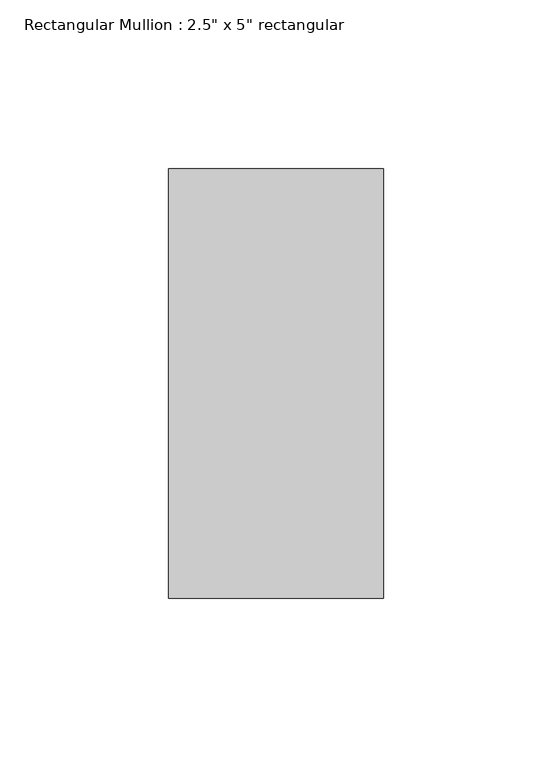
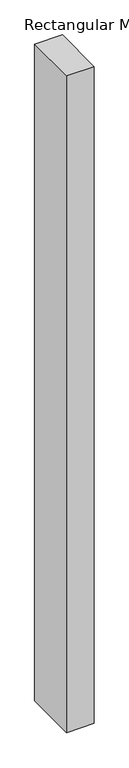
"""IFC4 building model written with IfcOpenShell, lengths in millimetres: member geometry."""

from ifc_helpers import new_model, si_unit, frame, origin, place, context, project, spatial, polyline, outline, extrude, source, transform, mapped, element, save


def member_001188f2(model_context):
    return source(origin(), model_context, "Body", "SweptSolid", [
        extrude(outline(polyline([(31.75, 63.5), (31.75, -63.5), (-31.75, -63.5), (-31.75, 63.5), (31.75, 63.5)])), frame((0.0, 0.0, -1599.2829369), z_axis=(0.0, 0.0, 1.0), x_axis=(1.0, 0.0, 0.0)), (0.0, 0.0, 1.0), 1599.2829369),
    ])


if __name__ == "__main__":
    model = new_model("IFC4")
    model_context = context("Model", 3, world=origin())
    ifc_project = project(units=[si_unit("LENGTHUNIT", "METRE", prefix="MILLI")], contexts=[model_context])
    site = spatial("IfcSite", under=ifc_project)
    building = spatial("IfcBuilding", under=site)
    placement = place(None, origin())
    member_shape = member_001188f2(model_context)
    element("IfcMember", 1, ObjectType="Rectangular Mullion : 2.5\" x 5\" rectangular", at=placement, inside=building, context=model_context, shape_type="MappedRepresentation", body=[
        mapped(member_shape, transform((0.0, 0.0, 0.0), x_axis=(1.0, 0.0, 0.0), y_axis=(0.0, 1.0, 0.0), z_axis=(0.0, 0.0, 1.0))),
    ])
    save(model, "model.ifc")

# Revit data of these elements
# Type "Rectangular Mullion : 2.5\" x 5\" rectangular"
#   built-in parameter 1007304 = 0.416667 (stored number, unit not read)
#   built-in parameter 1007301 = 0.104167 (stored number, unit not read)
#   built-in parameter 1007300 = 0.104167 (stored number, unit not read)
# Element 1 (IfcMember, "Rectangular Mullion : 2.5\" x 5\" rectangular")
#   Materials on its faces: "Aluminum"
# Materials
#   "Aluminum": class "Metal", colour RGB 247 247 247, transparency 0, Description = "Aluminum 6061", Cost = 0
